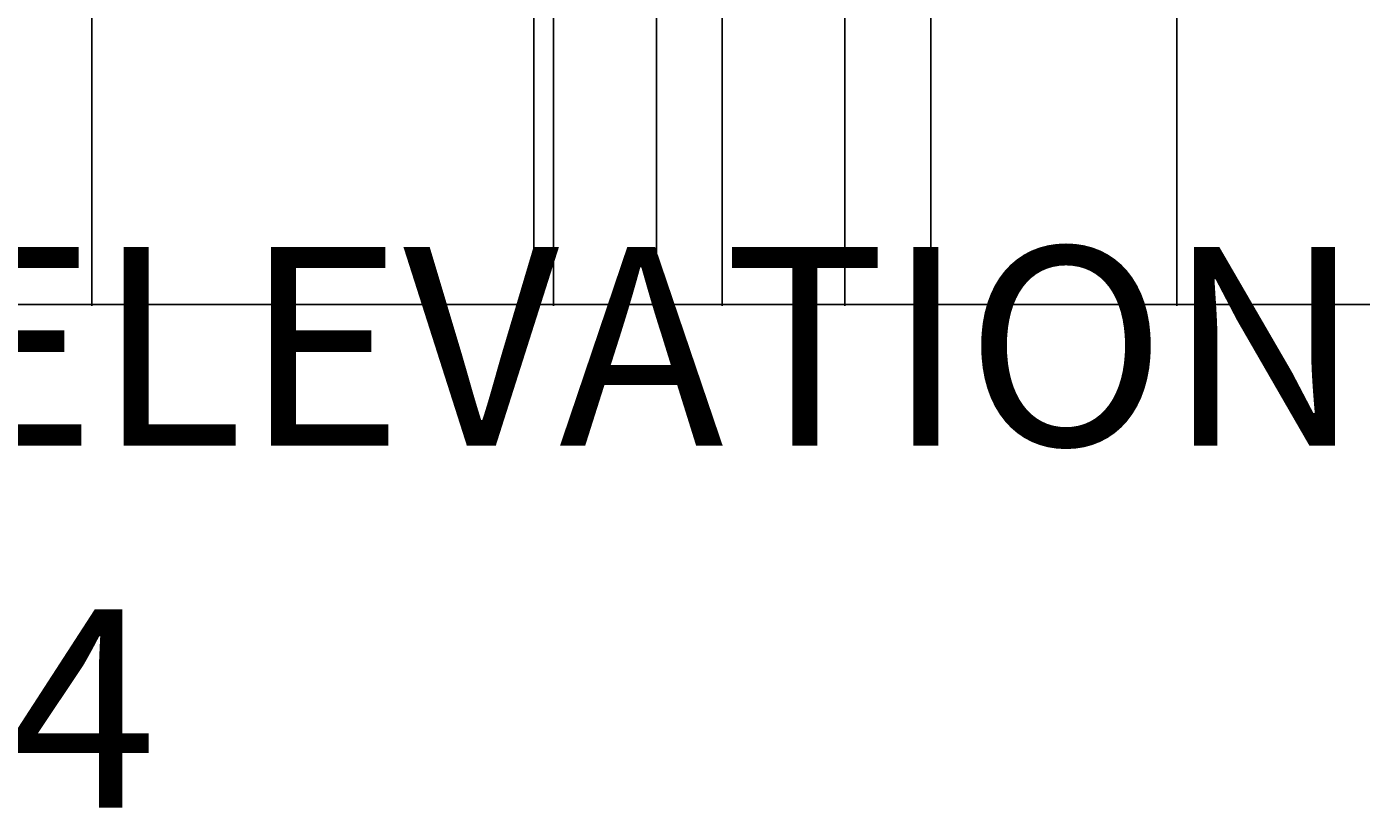
# Model space of a CAD drawing. Units: inches. Extents: x -15 to 605, y -220 to 570.
# Tile 3 of 10: x 265 to 438, y -220 to -118. Entities that reach past the tile are written whole.
import ezdxf

# ---------------------------------------------------------------- set-up
doc = ezdxf.new("R2010")
doc.units = ezdxf.units.IN
doc.header["$MEASUREMENT"] = 0
doc.layers.add('A-ANNO-DIMS', color=2, linetype='Continuous', lineweight=18)
doc.layers.add('A-ANNO-TEXT', color=7, linetype='Continuous', lineweight=25)
doc.styles.get("Standard").update_dxf_attribs({"font": 'arial.ttf'})
doc.dimstyles.get("Standard").update_dxf_attribs({"dimtxt": 0.18, "dimasz": 0.18, "dimexe": 0.18, "dimexo": 0.0625, "dimgap": 0.09, "dimtad": 0, "dimtih": 1, "dimtoh": 1, "dimdec": 4, "dimzin": 0, "dimdsep": 46, "dimtxsty": 'Standard', "dimcen": 0.09, "dimadec": 0, "dimazin": 0, "dimtfac": 1, "dimtdec": 4, "dimtofl": 0, "dimtmove": 0, "dimatfit": 3, "dimfxl": 1, "dimtolj": 1, "dimtzin": 0, "dimarcsym": 0})

# ---------------------------------------------------------------- blocks, each defined once
blk = doc.blocks.new('*D7')
at = {"layer": 'A-ANNO-DIMS', "color": 0, "lineweight": -2, "transparency": 16777216}
for p, q in [((23.99, 3.76), (23.99, -154.76)), ((566.72, -116.24), (566.72, -154.76)), ((24.17, -154.58), (294.96, -154.58)), ((566.54, -154.58), (295.75, -154.58))]:
    blk.add_line(p, q, dxfattribs=at)
at = {"layer": 'A-ANNO-DIMS', "color": 0, "transparency": 16777216}
for points in [[(24.17, -154.55), (24.17, -154.61), (23.99, -154.58)], [(566.54, -154.55), (566.54, -154.61), (566.72, -154.58)]]:
    blk.add_solid(points, dxfattribs=at)
at = {"layer": 'Defpoints', "color": 0, "transparency": 16777216}
for p in [(23.99, 3.82), (566.72, -116.18), (566.72, -154.58)]:
    blk.add_point(p, dxfattribs=at)
at = {"layer": 'A-ANNO-DIMS', "color": 0, "transparency": 16777216, "insert": (295.35, -154.58), "char_height": 0.18, "attachment_point": 5}
blk.add_mtext('\\A1;542.7', dxfattribs=at)
blk = doc.blocks.new('*D28')
at = {"layer": 'A-ANNO-DIMS', "color": 0, "lineweight": -2, "transparency": 16777216}
for p, q in [((260.99, 15.76), (260.99, -154.76)), ((272.99, 15.76), (272.99, -154.76)), ((261.17, -154.58), (266.78, -154.58)), ((272.81, -154.58), (267.2, -154.58))]:
    blk.add_line(p, q, dxfattribs=at)
at = {"layer": 'A-ANNO-DIMS', "color": 0, "transparency": 16777216}
for points in [[(261.17, -154.55), (261.17, -154.61), (260.99, -154.58)], [(272.81, -154.55), (272.81, -154.61), (272.99, -154.58)]]:
    blk.add_solid(points, dxfattribs=at)
at = {"layer": 'Defpoints', "color": 0, "transparency": 16777216}
for p in [(260.99, 15.82), (272.99, 15.82), (272.99, -154.58)]:
    blk.add_point(p, dxfattribs=at)
at = {"layer": 'A-ANNO-DIMS', "color": 0, "transparency": 16777216, "insert": (266.99, -154.58), "char_height": 0.18, "attachment_point": 5}
blk.add_mtext('\\A1;12', dxfattribs=at)
blk = doc.blocks.new('*D29')
at = {"layer": 'A-ANNO-DIMS', "color": 0, "lineweight": -2, "transparency": 16777216}
for p, q in [((272.99, 15.76), (272.99, -154.76)), ((332.99, 15.76), (332.99, -154.76)), ((273.17, -154.58), (302.77, -154.58)), ((332.81, -154.58), (303.21, -154.58))]:
    blk.add_line(p, q, dxfattribs=at)
at = {"layer": 'A-ANNO-DIMS', "color": 0, "transparency": 16777216}
for points in [[(273.17, -154.55), (273.17, -154.61), (272.99, -154.58)], [(332.81, -154.55), (332.81, -154.61), (332.99, -154.58)]]:
    blk.add_solid(points, dxfattribs=at)
at = {"layer": 'Defpoints', "color": 0, "transparency": 16777216}
for p in [(272.99, 15.82), (332.99, 15.82), (332.99, -154.58)]:
    blk.add_point(p, dxfattribs=at)
at = {"layer": 'A-ANNO-DIMS', "color": 0, "transparency": 16777216, "insert": (302.99, -154.58), "char_height": 0.18, "attachment_point": 5}
blk.add_mtext('\\A1;60', dxfattribs=at)
blk = doc.blocks.new('*D30')
at = {"layer": 'A-ANNO-DIMS', "color": 0, "lineweight": -2, "transparency": 16777216}
for p, q in [((382.03, 34.31), (382.03, -154.76)), ((332.99, 15.76), (332.99, -154.76)), ((333.17, -154.58), (357.11, -154.58)), ((381.85, -154.58), (357.91, -154.58))]:
    blk.add_line(p, q, dxfattribs=at)
at = {"layer": 'A-ANNO-DIMS', "color": 0, "transparency": 16777216}
for points in [[(333.17, -154.55), (333.17, -154.61), (332.99, -154.58)], [(381.85, -154.55), (381.85, -154.61), (382.03, -154.58)]]:
    blk.add_solid(points, dxfattribs=at)
at = {"layer": 'Defpoints', "color": 0, "transparency": 16777216}
for p in [(382.03, 34.38), (332.99, 15.82), (382.03, -154.58)]:
    blk.add_point(p, dxfattribs=at)
at = {"layer": 'A-ANNO-DIMS', "color": 0, "transparency": 16777216, "insert": (357.51, -154.58), "char_height": 0.18, "attachment_point": 5}
blk.add_mtext('\\A1;49.04', dxfattribs=at)
blk = doc.blocks.new('*D31')
at = {"layer": 'A-ANNO-DIMS', "color": 0, "lineweight": -2, "transparency": 16777216}
for p, q in [((382.03, 34.31), (382.03, -154.76)), ((491.99, 15.76), (491.99, -154.76)), ((382.21, -154.58), (436.55, -154.58)), ((491.81, -154.58), (437.46, -154.58))]:
    blk.add_line(p, q, dxfattribs=at)
at = {"layer": 'A-ANNO-DIMS', "color": 0, "transparency": 16777216}
for points in [[(382.21, -154.55), (382.21, -154.61), (382.03, -154.58)], [(491.81, -154.55), (491.81, -154.61), (491.99, -154.58)]]:
    blk.add_solid(points, dxfattribs=at)
at = {"layer": 'Defpoints', "color": 0, "transparency": 16777216}
for p in [(382.03, 34.38), (491.99, 15.82), (491.99, -154.58)]:
    blk.add_point(p, dxfattribs=at)
at = {"layer": 'A-ANNO-DIMS', "color": 0, "transparency": 16777216, "insert": (437.01, -154.58), "char_height": 0.18, "attachment_point": 5}
blk.add_mtext('\\A1;109.96', dxfattribs=at)
blk = doc.blocks.new('*D46')
at = {"layer": 'A-ANNO-DIMS', "color": 0, "lineweight": -2, "transparency": 16777216}
for p, q in [((251.99, -116.24), (251.99, -154.76)), ((330.43, -116.24), (330.43, -154.76)), ((252.17, -154.58), (290.82, -154.58)), ((330.25, -154.58), (291.6, -154.58))]:
    blk.add_line(p, q, dxfattribs=at)
at = {"layer": 'A-ANNO-DIMS', "color": 0, "transparency": 16777216}
for points in [[(252.17, -154.55), (252.17, -154.61), (251.99, -154.58)], [(330.25, -154.55), (330.25, -154.61), (330.43, -154.58)]]:
    blk.add_solid(points, dxfattribs=at)
at = {"layer": 'Defpoints', "color": 0, "transparency": 16777216}
for p in [(251.99, -116.18), (330.43, -116.18), (330.43, -154.58)]:
    blk.add_point(p, dxfattribs=at)
at = {"layer": 'A-ANNO-DIMS', "color": 0, "transparency": 16777216, "insert": (291.21, -154.58), "char_height": 0.18, "attachment_point": 5}
blk.add_mtext('\\A1;78.45', dxfattribs=at)
blk = doc.blocks.new('*D47')
at = {"layer": 'A-ANNO-DIMS', "color": 0, "lineweight": -2, "transparency": 16777216}
for p, q in [((330.43, -116.24), (330.43, -154.76)), ((346.37, -116.24), (346.37, -154.76)), ((330.61, -154.58), (337.94, -154.58)), ((346.19, -154.58), (338.85, -154.58))]:
    blk.add_line(p, q, dxfattribs=at)
at = {"layer": 'A-ANNO-DIMS', "color": 0, "transparency": 16777216}
for points in [[(330.61, -154.55), (330.61, -154.61), (330.43, -154.58)], [(346.19, -154.55), (346.19, -154.61), (346.37, -154.58)]]:
    blk.add_solid(points, dxfattribs=at)
at = {"layer": 'Defpoints', "color": 0, "transparency": 16777216}
for p in [(330.43, -116.18), (346.37, -116.18), (346.37, -154.58)]:
    blk.add_point(p, dxfattribs=at)
at = {"layer": 'A-ANNO-DIMS', "color": 0, "transparency": 16777216, "insert": (338.4, -154.58), "char_height": 0.18, "attachment_point": 5}
blk.add_mtext('\\A1;15.934', dxfattribs=at)
blk = doc.blocks.new('*D48')
at = {"layer": 'A-ANNO-DIMS', "color": 0, "lineweight": -2, "transparency": 16777216}
for p, q in [((346.37, -116.24), (346.37, -154.76)), ((354.92, -116.24), (354.92, -154.76)), ((346.55, -154.58), (350.32, -154.58)), ((354.74, -154.58), (350.97, -154.58))]:
    blk.add_line(p, q, dxfattribs=at)
at = {"layer": 'A-ANNO-DIMS', "color": 0, "transparency": 16777216}
for points in [[(346.55, -154.55), (346.55, -154.61), (346.37, -154.58)], [(354.74, -154.55), (354.74, -154.61), (354.92, -154.58)]]:
    blk.add_solid(points, dxfattribs=at)
at = {"layer": 'Defpoints', "color": 0, "transparency": 16777216}
for p in [(346.37, -116.18), (354.92, -116.18), (354.92, -154.58)]:
    blk.add_point(p, dxfattribs=at)
at = {"layer": 'A-ANNO-DIMS', "color": 0, "transparency": 16777216, "insert": (350.64, -154.58), "char_height": 0.18, "attachment_point": 5}
blk.add_mtext('\\A1;8.55', dxfattribs=at)
blk = doc.blocks.new('*D49')
at = {"layer": 'A-ANNO-DIMS', "color": 0, "lineweight": -2, "transparency": 16777216}
for p, q in [((354.92, -116.24), (354.92, -154.76)), ((370.85, -116.24), (370.85, -154.76)), ((355.1, -154.58), (362.43, -154.58)), ((370.67, -154.58), (363.34, -154.58))]:
    blk.add_line(p, q, dxfattribs=at)
at = {"layer": 'A-ANNO-DIMS', "color": 0, "transparency": 16777216}
for points in [[(355.1, -154.55), (355.1, -154.61), (354.92, -154.58)], [(370.67, -154.55), (370.67, -154.61), (370.85, -154.58)]]:
    blk.add_solid(points, dxfattribs=at)
at = {"layer": 'Defpoints', "color": 0, "transparency": 16777216}
for p in [(354.92, -116.18), (370.85, -116.18), (370.85, -154.58)]:
    blk.add_point(p, dxfattribs=at)
at = {"layer": 'A-ANNO-DIMS', "color": 0, "transparency": 16777216, "insert": (362.88, -154.58), "char_height": 0.18, "attachment_point": 5}
blk.add_mtext('\\A1;15.934', dxfattribs=at)
blk = doc.blocks.new('*D50')
at = {"layer": 'A-ANNO-DIMS', "color": 0, "lineweight": -2, "transparency": 16777216}
for p, q in [((370.85, -116.24), (370.85, -154.76)), ((414, -116.24), (414, -154.76)), ((371.03, -154.58), (392.03, -154.58)), ((413.82, -154.58), (392.82, -154.58))]:
    blk.add_line(p, q, dxfattribs=at)
at = {"layer": 'A-ANNO-DIMS', "color": 0, "transparency": 16777216}
for points in [[(371.03, -154.55), (371.03, -154.61), (370.85, -154.58)], [(413.82, -154.55), (413.82, -154.61), (414, -154.58)]]:
    blk.add_solid(points, dxfattribs=at)
at = {"layer": 'Defpoints', "color": 0, "transparency": 16777216}
for p in [(370.85, -116.18), (414, -116.18), (414, -154.58)]:
    blk.add_point(p, dxfattribs=at)
at = {"layer": 'A-ANNO-DIMS', "color": 0, "transparency": 16777216, "insert": (392.42, -154.58), "char_height": 0.18, "attachment_point": 5}
blk.add_mtext('\\A1;43.15', dxfattribs=at)
blk = doc.blocks.new('*D51')
at = {"layer": 'A-ANNO-DIMS', "color": 0, "lineweight": -2, "transparency": 16777216}
for p, q in [((414, -116.24), (414, -154.76)), ((566.72, -116.24), (566.72, -154.76)), ((414.18, -154.58), (489.9, -154.58)), ((566.54, -154.58), (490.81, -154.58))]:
    blk.add_line(p, q, dxfattribs=at)
at = {"layer": 'A-ANNO-DIMS', "color": 0, "transparency": 16777216}
for points in [[(414.18, -154.55), (414.18, -154.61), (414, -154.58)], [(566.54, -154.55), (566.54, -154.61), (566.72, -154.58)]]:
    blk.add_solid(points, dxfattribs=at)
at = {"layer": 'Defpoints', "color": 0, "transparency": 16777216}
for p in [(414, -116.18), (566.72, -116.18), (566.72, -154.58)]:
    blk.add_point(p, dxfattribs=at)
at = {"layer": 'A-ANNO-DIMS', "color": 0, "transparency": 16777216, "insert": (490.36, -154.58), "char_height": 0.18, "attachment_point": 5}
blk.add_mtext('\\A1;152.72', dxfattribs=at)

msp = doc.modelspace()

# ---------------------------------------------------------------- texts
at = {"layer": 'A-ANNO-TEXT'}
for s, height, p in [('FRONT ELEVATION', 25.818282, (130.4215, -172.9392)), ('G+4', 25.81828, (218.0971, -220.0392))]:
    msp.add_text(s, height=height, dxfattribs=at).set_placement(p)

# ---------------------------------------------------------------- dimensions: what is measured, and where the dimension line sits
at = {"layer": 'A-ANNO-DIMS'}
for base, p1, p2, override, picture, middle in [((382.0304, -154.5813), (332.9872, 15.8187), (382.0304, 34.3758), {"dimdec": 2, "dimlfac": 1, "dimrnd": 0, "dimzin": 0, "dimdsep": 46, "dimlunit": 2}, '*D30', (357.5088, -154.5813)), ((491.9872, -154.5813), (382.0304, 34.3758), (491.9872, 15.8187), {"dimdec": 2, "dimlfac": 1, "dimrnd": 0, "dimzin": 0, "dimdsep": 46, "dimlunit": 2}, '*D31', (437.0088, -154.5813)), ((272.9872, -154.5813), (260.9872, 15.8187), (272.9872, 15.8187), {"dimdec": 0, "dimlfac": 1, "dimrnd": 0, "dimzin": 0, "dimdsep": 46, "dimlunit": 2}, '*D28', (266.9872, -154.5813)), ((332.9872, -154.5813), (272.9872, 15.8187), (332.9872, 15.8187), {"dimdec": 0, "dimlfac": 1, "dimrnd": 0, "dimzin": 0, "dimdsep": 46, "dimlunit": 2}, '*D29', (302.9872, -154.5813)), ((566.7161, -154.5813), (23.9872, 3.8187), (566.7161, -116.1813), {"dimdec": 1, "dimlfac": 1, "dimrnd": 0, "dimzin": 0, "dimdsep": 46, "dimlunit": 2}, '*D7', (295.3517, -154.5813)), ((330.4327, -154.5813), (251.9872, -116.1813), (330.4327, -116.1813), {"dimdec": 2, "dimlfac": 1, "dimrnd": 0, "dimzin": 0, "dimdsep": 46, "dimlunit": 2}, '*D46', (291.21, -154.5813)), ((346.3663, -154.5813), (330.4327, -116.1813), (346.3663, -116.1813), {"dimdec": 3, "dimlfac": 1, "dimrnd": 0, "dimzin": 0, "dimdsep": 46, "dimlunit": 2}, '*D47', (338.3995, -154.5813)), ((354.916, -154.5813), (346.3663, -116.1813), (354.916, -116.1813), {"dimdec": 2, "dimlfac": 1, "dimrnd": 0, "dimzin": 0, "dimdsep": 46, "dimlunit": 2}, '*D48', (350.6411, -154.5813)), ((370.8496, -154.5813), (354.916, -116.1813), (370.8496, -116.1813), {"dimdec": 3, "dimlfac": 1, "dimrnd": 0, "dimzin": 0, "dimdsep": 46, "dimlunit": 2}, '*D49', (362.8828, -154.5813)), ((413.9976, -154.5813), (370.8496, -116.1813), (413.9976, -116.1813), {"dimdec": 2, "dimlfac": 1, "dimrnd": 0, "dimzin": 0, "dimdsep": 46, "dimlunit": 2}, '*D50', (392.4236, -154.5813)), ((566.7161, -154.5813), (413.9976, -116.1813), (566.7161, -116.1813), {"dimdec": 2, "dimlfac": 1, "dimrnd": 0, "dimzin": 0, "dimdsep": 46, "dimlunit": 2}, '*D51', (490.3568, -154.5813))]:
    dim = msp.add_linear_dim(base=base, p1=p1, p2=p2, dimstyle='Standard', override=override, dxfattribs=at)
    dim.commit()
    dim.dimension.update_dxf_attribs({"geometry": picture, "text_midpoint": middle})

doc.saveas('drawing.dxf')
